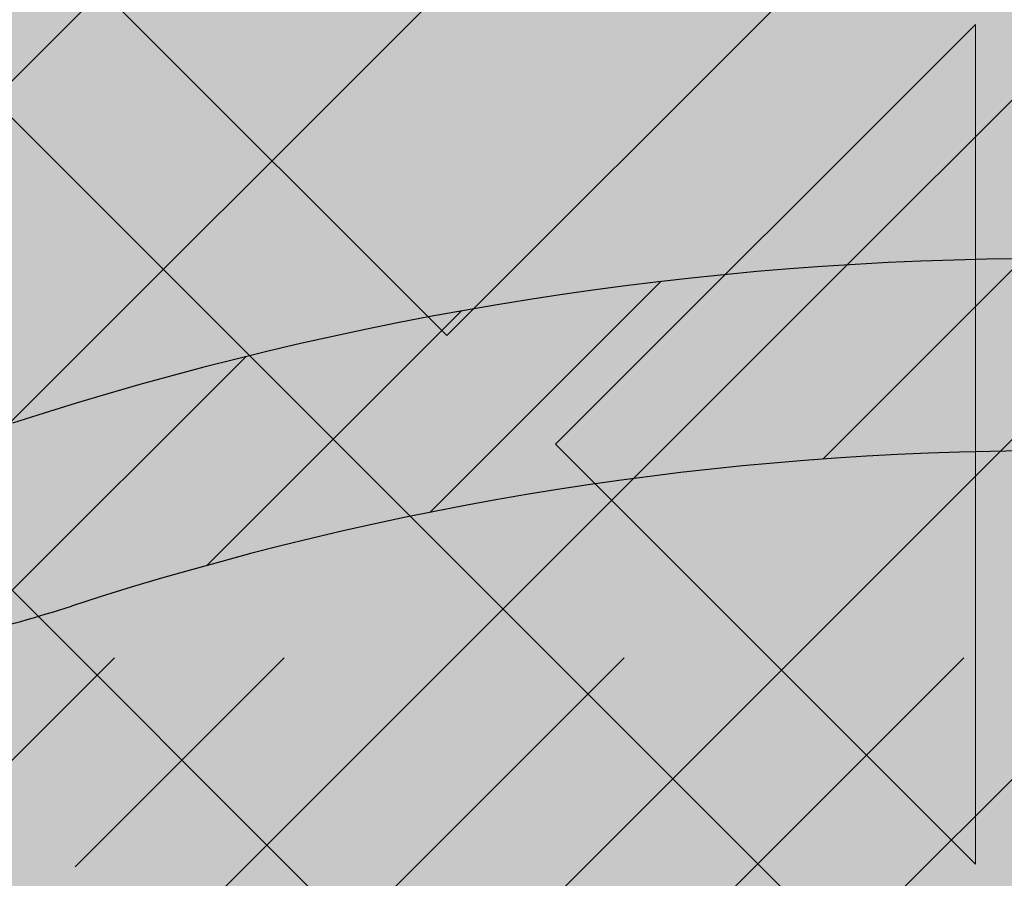
# Model space of a CAD drawing. Units: inches. Extents: x 844 to 2234, y 346 to 1084.
# Tile 20 of 93: x 1121.143 to 1122.777, y 702.178 to 703.603. Entities that reach past the tile are written whole.
import ezdxf

# ---------------------------------------------------------------- set-up
doc = ezdxf.new("R2010")
doc.units = ezdxf.units.IN
doc.header["$MEASUREMENT"] = 0
for name, color, linetype, lineweight in [('A-ANNO-DIMS', 2, 'Continuous', 18), ('furniture', 8, 'Continuous', 18), ('RA-AP-01$0$INT', 35, 'Continuous', 5)]:
    doc.layers.add(name, color=color, linetype=linetype, lineweight=lineweight)
doc.layers.add('RA-AP-01$0$FURN', color=3, linetype='Continuous')
doc.layers.add('RA-AP-01$0$WOOD', color=64, linetype='Continuous')
doc.styles.get("Standard").update_dxf_attribs({"font": 'arial.ttf'})
doc.dimstyles.get("Standard").update_dxf_attribs({"dimtxt": 6, "dimasz": 3, "dimexe": 0.18, "dimexo": 0.0625, "dimgap": 0.09, "dimtad": 0, "dimtih": 1, "dimtoh": 1, "dimdec": 1, "dimzin": 0, "dimdsep": 46, "dimlunit": 3, "dimtxsty": 'Standard', "dimblk": 'ARCHTICK', "dimcen": 0.09, "dimadec": 0, "dimazin": 0, "dimtfac": 1, "dimtdec": 1, "dimtofl": 0, "dimtmove": 0, "dimatfit": 3, "dimfxl": 1, "dimtolj": 1, "dimtzin": 0, "dimarcsym": 0})

# ---------------------------------------------------------------- blocks, each defined once
blk = doc.blocks.new('A$C18D01794')
at = {"layer": 'RA-AP-01$0$INT'}
h = blk.add_hatch(color=256, dxfattribs=at)
h.paths.add_polyline_path([(4.585917135068448, -7.856712009587804), (4.614201406330596, -7.856712009587056), (4.668846067270487, -7.802067348644738), (4.723490728212344, -7.856712009584164), (4.771774999457151, -7.856712009582887), (4.826419660396886, -7.80206734864072), (4.862780050090322, -7.838427738332541), (4.844495778842715, -7.856712009580965), (4.862780050090411, -7.856712009580482), (4.905206456960182, -7.814285602707865), (4.947632863832445, -7.856712009578238), (4.965917135079675, -7.856712009577755), (4.947632863831759, -7.838427738330656), (4.983993253523576, -7.802067348637219), (5.038637914464627, -7.856712009575829), (5.08692218571208, -7.856712009574554), (5.141566846649976, -7.802067348634224), (5.196211507589851, -7.856712009571666), (5.224495778822615, -7.856712009570916), (4.905206456953975, -7.537422687702283)])
h.paths.add_polyline_path([(4.895206456956031, -7.575706958950402), (4.895206456958921, -7.684996280828174), (4.840561796018589, -7.630351619890275)], flags=16)
h.paths.add_polyline_path([(4.915206456955638, -7.575706958949956), (4.969851117895509, -7.630351619887399), (4.915206456957609, -7.684996280827732)], flags=16)
h.paths.add_polyline_path([(4.826419660395175, -7.644493755514321), (4.881064321335613, -7.699138416452331), (4.771774999456703, -7.69913841645522)], flags=16)
h.paths.add_polyline_path([(4.983993253519558, -7.644493755510815), (5.038637914460456, -7.699138416449285), (4.929348592581548, -7.69913841645126)], flags=16)
h.paths.add_polyline_path([(4.881064321336025, -7.719138416452334), (4.826419660397532, -7.773783077393256), (4.771774999457062, -7.719138416455217)], flags=16)
h.paths.add_polyline_path([(4.929348592582019, -7.71913841645126), (5.038637914460982, -7.719138416449284), (4.983993253522945, -7.773783077389749)], flags=16)
h.paths.add_polyline_path([(4.895206456960191, -7.733280552075633), (4.895206456962115, -7.806001331460164), (4.876922185715016, -7.824285602708492), (4.840561796021581, -7.787925213016675)], flags=16)
h.paths.add_polyline_path([(4.915206456958487, -7.733280552075187), (4.969851117899527, -7.787925213013798), (4.933490728206909, -7.824285602708034), (4.9152064569598, -7.806001331461736)], flags=16)
h.paths.add_polyline_path([(4.757632863832376, -7.733280552079264), (4.812277524772842, -7.787925213017304), (4.757632863834348, -7.842569873958233)], flags=16)
h.paths.add_polyline_path([(4.737632863832376, -7.73328055207979), (4.737632863834348, -7.842569873958701), (4.682988202893906, -7.787925213020692)], flags=16)
h.paths.add_polyline_path([(5.05278005008503, -7.733280552072701), (5.052780050087917, -7.842569873951664), (4.998135389146995, -7.787925213013169)], flags=16)
h.paths.add_polyline_path([(5.072780050085024, -7.733280552072333), (5.127424711025931, -7.787925213010806), (5.072780050087916, -7.842569873951244)], flags=16)
h.paths.add_polyline_path([(4.935917135072783, -7.506712009583784), (5.255206456948811, -7.826001331459767), (5.255206456948932, -7.797717060211899), (5.200561796010279, -7.743072399273238), (5.255206456949403, -7.688427738334128), (5.25520645694961, -7.640143467086677), (5.200561796009787, -7.585498806146837), (5.236922185702417, -7.549138416454212), (5.255206456949919, -7.56742268770172), (5.255206456949998, -7.549138416454178), (5.212780050078687, -7.506712009583814), (5.25520645695036, -7.464285602712145), (5.255206456950438, -7.446001331464763), (5.236922185702424, -7.464285602712779), (5.200561796009796, -7.427925213020149), (5.255206456950753, -7.373280552079203), (5.25520645695096, -7.324996280834394), (5.200561796010322, -7.270351619893748), (5.255206456951428, -7.215706958952649), (5.255206456951547, -7.187422687705071)])
h.paths.add_polyline_path([(5.042988202883395, -7.42792521302065), (5.097632863823085, -7.373280552080975), (5.097632863822622, -7.482569873959883)], flags=16)
h.paths.add_polyline_path([(5.028846067259663, -7.442067348644384), (5.083490728198774, -7.496712009583504), (4.974201406321001, -7.496712009583035)], flags=16)
h.paths.add_polyline_path([(5.117632863823087, -7.37328055208089), (5.172277524762331, -7.42792521302015), (5.11763286382262, -7.482569873959851)], flags=16)
h.paths.add_polyline_path([(5.08349072819877, -7.516712009582191), (5.028846067259652, -7.571356670521302), (4.974201406320998, -7.516712009582638)], flags=16)
h.paths.add_polyline_path([(5.131774999446817, -7.35913841645716), (5.186419660386065, -7.413783077396415), (5.241064321325782, -7.359138416456712)], flags=17)
h.paths.add_polyline_path([(5.131774999446228, -7.496712009583703), (5.186419660386065, -7.442067348643883), (5.222780050079488, -7.478427738337313), (5.204495778832781, -7.496712009584014)], flags=16)
h.paths.add_polyline_path([(5.097632863822613, -7.530854145205813), (5.097632863823061, -7.640143467084723), (5.042988202883383, -7.585498806145032)], flags=16)
h.paths.add_polyline_path([(5.131774999446899, -7.339138416457162), (5.241064321325809, -7.339138416456712), (5.186419660386591, -7.284493755517479)], flags=17)
h.paths.add_polyline_path([(5.131774999446226, -7.516712009581999), (5.204495778830767, -7.516712009581702), (5.22278005007868, -7.534996280829206), (5.186419660386049, -7.571356670521828)], flags=16)
h.paths.add_polyline_path([(5.11763286382262, -7.530854145205852), (5.17227752476232, -7.585498806145562), (5.117632863823064, -7.64014346708481)], flags=16)
h.paths.add_polyline_path([(5.186419660386069, -7.599640941770585), (5.241064321325754, -7.654285602710281), (5.131774999446791, -7.654285602709814)], flags=16)
h.paths.add_polyline_path([(5.131774999446872, -7.674285602709813), (5.24106432132578, -7.674285602710282), (5.186419660386554, -7.728930263649504)], flags=16)
h.paths.add_polyline_path([(5.255206456951811, -7.126001331467467), (5.255206456951895, -7.106712009588038), (4.555206456956052, -7.106712009588038), (4.555206456956136, -7.12600133146746), (4.905206456953973, -7.476001331465289)])
h.paths.add_polyline_path([(4.983993253513404, -7.368930263651977), (4.92934859257295, -7.314285602713969), (5.03863791445186, -7.314285602711063)], flags=16)
h.paths.add_polyline_path([(4.969851117889988, -7.383072399276016), (4.915206456952556, -7.437717060215906), (4.915206456949648, -7.328427738338133)], flags=16)
h.paths.add_polyline_path([(4.929348592572535, -7.294285602713971), (4.983993253511019, -7.239640941773039), (5.038637914451496, -7.294285602711065)], flags=16)
h.paths.add_polyline_path([(5.052780050074912, -7.280143467087016), (4.998135389134438, -7.225498806148989), (5.052780050072919, -7.170854145208052)], flags=16)
h.paths.add_polyline_path([(5.07278005007491, -7.280143467086489), (5.072780050072918, -7.170854145207579), (5.127424711013374, -7.225498806145578)], flags=16)
h.paths.add_polyline_path([(4.89520645695295, -7.437717060216355), (4.840561796013067, -7.383072399278919), (4.895206456950961, -7.328427738338582)], flags=16)
h.paths.add_polyline_path([(4.915206456948365, -7.280143467090674), (4.915206456946434, -7.207422687704125), (4.933490728192729, -7.18913841645701), (4.969851117886972, -7.225498806149623)], flags=16)
h.paths.add_polyline_path([(4.881064321327021, -7.314285602715054), (4.82641966038902, -7.368930263655506), (4.771774999448108, -7.314285602717047)], flags=16)
h.paths.add_polyline_path([(4.895206456950073, -7.280143467091125), (4.840561796009022, -7.225498806152518), (4.876922185700835, -7.18913841645908), (4.895206456948749, -7.207422687706589)], flags=16)
h.paths.add_polyline_path([(4.983993253510392, -7.211356670525576), (4.947632863816944, -7.174996280833758), (4.965917135064043, -7.156712009585847), (5.038637914448995, -7.156712009584522)], flags=16)
h.paths.add_polyline_path([(4.881064321326543, -7.294285602715056), (4.771774999447578, -7.294285602717046), (4.826419660385607, -7.239640941776569)], flags=16)
h.paths.add_polyline_path([(4.905206456946447, -7.19913841645844), (4.862780050074785, -7.156712009587725), (4.947632863816685, -7.156712009586302)], flags=16)
h.paths.add_polyline_path([(5.14156684663679, -7.211356670521528), (5.086922185696452, -7.156712009583639), (5.196211507574223, -7.156712009581651)], flags=16)
h.paths.add_polyline_path([(4.8264196603837, -7.211356670529104), (4.771774999442643, -7.156712009590501), (4.8444957788276, -7.156712009588568), (4.862780050075511, -7.17499628083566)], flags=16)
h.paths.add_polyline_path([(4.812277524760289, -7.225498806153156), (4.757632863822258, -7.28014346709363), (4.757632863819352, -7.170854145214669)], flags=16)
h.paths.add_polyline_path([(4.73763286382226, -7.280143467093997), (4.682988202881349, -7.22549880615554), (4.737632863819352, -7.170854145215086)], flags=16)
h.paths.add_polyline_path([(4.723490728195188, -7.156712009591787), (4.668846067257299, -7.211356670532127), (4.614201406317417, -7.156712009594693)], flags=16)
h.paths.add_polyline_path([(4.597632863829262, -7.506712009583814), (4.555206456957951, -7.54913841645418), (4.555206456958029, -7.56742268770172), (4.573490728205535, -7.549138416454212), (4.609851117898167, -7.585498806146839), (4.555206456958338, -7.640143467086675), (4.555206456958546, -7.688427738334125), (4.60985111789767, -7.743072399273238), (4.555206456959015, -7.797717060211899), (4.555206456959138, -7.826001331459767), (4.874495778835167, -7.506712009583786), (4.5552064569564, -7.187422687705062), (4.555206456956523, -7.215706958952644), (4.609851117897629, -7.270351619893746), (4.555206456956988, -7.324996280834396), (4.555206456957198, -7.373280552079195), (4.609851117898153, -7.427925213020147), (4.573490728205528, -7.464285602712779), (4.555206456957507, -7.446001331464756), (4.555206456957585, -7.464285602712143)])
h.paths.add_polyline_path([(4.712780050085332, -7.482569873959882), (4.712780050084863, -7.373280552080972), (4.767424711024555, -7.42792521302065)], flags=16)
h.paths.add_polyline_path([(4.726922185709173, -7.496712009583504), (4.781566846648288, -7.442067348644384), (4.836211507586949, -7.496712009583033)], flags=16)
h.paths.add_polyline_path([(4.692780050085327, -7.482569873959851), (4.638135389145619, -7.427925213020149), (4.692780050084865, -7.373280552080892)], flags=16)
h.paths.add_polyline_path([(4.726922185709182, -7.516712009582191), (4.836211507586949, -7.51671200958264), (4.7815668466483, -7.571356670521304)], flags=16)
h.paths.add_polyline_path([(4.678637914461726, -7.496712009583706), (4.605917135075169, -7.496712009584014), (4.587632863828464, -7.478427738337311), (4.623993253521887, -7.442067348643881)], flags=16)
h.paths.add_polyline_path([(4.712780050085336, -7.530854145205816), (4.767424711024568, -7.585498806145034), (4.71278005008489, -7.640143467084724)], flags=16)
h.paths.add_polyline_path([(4.678637914461726, -7.516712009582001), (4.623993253521899, -7.571356670521829), (4.587632863829271, -7.534996280829206), (4.605917135077185, -7.5167120095817)], flags=16)
h.paths.add_polyline_path([(4.692780050085336, -7.530854145205848), (4.692780050084889, -7.64014346708481), (4.638135389145632, -7.585498806145562)], flags=16)
h.paths.add_polyline_path([(4.623993253521885, -7.413783077396415), (4.678637914461131, -7.359138416457161), (4.56934859258217, -7.359138416456712)], flags=17)
h.paths.add_polyline_path([(4.623993253521901, -7.599640941770568), (4.678637914461158, -7.654285602709814), (4.569348592582195, -7.654285602710281)], flags=16)
h.paths.add_polyline_path([(4.678637914461051, -7.339138416457162), (4.623993253521361, -7.284493755517479), (4.569348592582143, -7.339138416456712)], flags=17)
h.paths.add_polyline_path([(4.678637914461076, -7.674285602709813), (4.623993253521399, -7.728930263649504), (4.569348592582167, -7.674285602710281)], flags=16)
h = blk.add_hatch(color=256, dxfattribs=at)
h.paths.add_polyline_path([(4.905206456954232, -7.537422687702028), (4.874495778835232, -7.506712009583718), (4.555206456959138, -7.826001331459766), (4.555206456959269, -7.856712009588616), (4.585917135068449, -7.856712009587804)])
h.paths.add_polyline_path([(4.935917135072152, -7.506712009583152), (4.905206456953497, -7.537422687701806), (5.224495778822614, -7.856712009570917), (5.255206456948681, -7.856712009570104), (5.255206456948813, -7.826001331459768)])
h.paths.add_polyline_path([(5.255206456951549, -7.18742268770507), (5.255206456951813, -7.126001331467461), (4.905206456953563, -7.476001331465701), (4.935917135072559, -7.506712009584006)])
h.paths.add_polyline_path([(4.874495778835167, -7.506712009583785), (4.905206456953818, -7.476001331465132), (4.555206456956135, -7.126001331467458), (4.555206456956399, -7.187422687705064)])
h = blk.add_hatch(color=256, dxfattribs=at)
h.paths.add_polyline_path([(4.969851117891331, -7.630351619889621), (4.915206456952669, -7.575706958950966), (4.915206456952222, -7.684996280828739)])
h.paths.add_polyline_path([(4.895206456953064, -7.575706958950968), (4.840561796014413, -7.630351619889628), (4.895206456953533, -7.684996280828741)])
h.paths.add_polyline_path([(4.826419660390684, -7.644493755513362), (4.771774999451003, -7.699138416453052), (4.881064321329913, -7.699138416452587)])
h.paths.add_polyline_path([(4.881064321329884, -7.719138416452585), (4.771774999450921, -7.719138416453052), (4.82641966039018, -7.773783077392298)])
h.paths.add_polyline_path([(4.895206456953734, -7.733280552076196), (4.840561796013912, -7.787925213016031), (4.876922185707337, -7.824285602709455), (4.895206456954043, -7.806001331462747)])
h.paths.add_polyline_path([(4.862780050082808, -7.838427738332388), (4.826419660390178, -7.802067348639763), (4.771774999450351, -7.856712009579595), (4.844495778835303, -7.856712009579895)])
h.paths.add_polyline_path([(4.812277524766446, -7.787925213016036), (4.757632863827191, -7.733280552076788), (4.757632863826741, -7.842569873955747)])
h.paths.add_polyline_path([(4.737632863827191, -7.733280552076863), (4.682988202887508, -7.787925213016558), (4.737632863826743, -7.842569873955778)])
h.paths.add_polyline_path([(4.668846067263777, -7.802067348640287), (4.614201406325123, -7.856712009578949), (4.723490728202894, -7.856712009579402)])
h.paths.add_polyline_path([(4.905206456953846, -7.814285602708654), (4.862780050082654, -7.856712009579847), (4.947632863824561, -7.85671200958032)])
h.paths.add_polyline_path([(4.915206456952028, -7.733280552076195), (4.91520645695173, -7.806001331460731), (4.933490728199234, -7.824285602708648), (4.96985111789186, -7.787925213016022)])
h.paths.add_polyline_path([(5.038637914454841, -7.719138416453029), (4.929348592575874, -7.71913841645258), (4.983993253515593, -7.773783077392289)])
h.paths.add_polyline_path([(4.983993253515065, -7.644493755513352), (4.929348592575849, -7.699138416452582), (5.038637914454755, -7.699138416453031)])
h.paths.add_polyline_path([(5.052780050079843, -7.73328055207676), (4.998135389140595, -7.787925213016018), (5.052780050080309, -7.842569873955721)])
h.paths.add_polyline_path([(4.983993253516868, -7.802067348639752), (4.947632863824241, -7.838427738332383), (4.965917135071747, -7.856712009579888), (5.038637914456701, -7.856712009579572)])
h.paths.add_polyline_path([(5.127424711019533, -7.787925213016519), (5.072780050079843, -7.733280552076838), (5.07278005008031, -7.842569873955751)])
h.paths.add_polyline_path([(5.141566846643269, -7.802067348640248), (5.086922185704154, -7.85671200957937), (5.196211507581929, -7.856712009578901)])
for p, q in [((4.874495778835167, -7.506712009583786), (4.555206456959136, -7.826001331459769)), ((4.905206456953975, -7.537422687702283), (4.585917135071132, -7.856712009585121)), ((4.895206456956031, -7.575706958950402), (4.840561796018589, -7.630351619890275)), ((4.895206456958921, -7.684996280828173), (4.895206456956031, -7.575706958950402)), ((4.895206456958917, -7.684996280828171), (4.840561796018589, -7.630351619890275)), ((4.826419660395171, -7.644493755514321), (4.771774999456703, -7.69913841645522)), ((4.881064321335613, -7.699138416452333), (4.826419660395173, -7.64449375551432))]:
    blk.add_line(p, q, dxfattribs=at)
blk = doc.blocks.new('A$C32926AE1')
at = {"layer": 'RA-AP-01$0$FURN'}
h = blk.add_hatch(dxfattribs=at)
h.set_pattern_fill('ANSI31', color=256, scale=0.1, style=0)
h.set_pattern_definition([(45, (0, 0), (-0.0088388347648318, 0.0088388347648318), [])])
edge = h.paths.add_edge_path(flags=16)
edge.add_arc((4.904771284329206, 4.246793130718756), 0.2603971832811541, 75.22398030683196, 104.7760196931204)
edge.add_arc((4.904771284329206, 4.246793130718756), 0.2603971832811541, 75.223980306832, 104.77601969312039, ccw=False)
edge = h.paths.add_edge_path(flags=16)
edge.add_arc((4.904771284329206, 4.067062675376612), 0.2603971832811541, 255.2239803068796, 284.776019693168)
edge.add_arc((4.904771284329206, 4.067062675376612), 0.2603971832811541, 255.22398030687958, 284.77601969316805, ccw=False)
edge = h.paths.add_edge_path(flags=0)
edge.add_arc((4.904771284329206, 4.067062675376612), 0.2603971832811541, 255.2239803068796, 284.776019693168)
edge.add_arc((4.904771284329206, 4.067062675376612), 0.2603971832811541, 255.22398030687958, 284.77601969316805, ccw=False)
edge = h.paths.add_edge_path(flags=0)
edge.add_arc((4.904771284329206, 4.067062675376612), 0.2603971832811541, 255.2239803068796, 284.776019693168)
edge.add_arc((4.904771284329206, 4.067062675376612), 0.2603971832811541, 255.22398030687958, 284.77601969316805, ccw=False)
edge = h.paths.add_edge_path()
edge.add_arc((4.604388392048174, 4.588829985554312), 0.1599999999999918, 342.3781640246255, 354.4317409793762)
edge.add_arc((5.090145208887507, 4.43216705527679), 0.3503971832811637, 162.0091218307731, 180.3186872093483)
edge.add_arc((5.205154176610243, 4.588829985554953), 0.1599999999999917, 185.5682590208461, 197.6218359767349)
edge.add_arc((4.904771284329229, 4.246793130718735), 0.3503971832811761, 72.00912183053516, 107.9908781690354)
edge.add_arc((9.535952835716557, 4.28682295566602), 4.798342501046485, 178.2875002453811, 181.5576802719453)
edge.add_arc((4.719397359771122, 4.43216705527679), 0.3503971832811637, 359.6813127906516, 377.9908781692269)
edge.add_arc((9.535967292294904, 4.286822350292874), 4.778371420254705, 178.2965938931842, 181.5667745797229)
edge.add_arc((4.719397359771122, 4.43216705527679), 0.3303971832811637, 359.6813127906516, 377.9908781692269)
edge.add_arc((0.2735752763637294, 4.286822350292874), 4.7783714202547, 358.4332254202771, 361.7034061068158)
edge.add_arc((5.061434214606998, 4.732549947558029), 0.1600000000000254, 252.3781640250584, 264.4317409792362)
edge.add_arc((4.748108354051257, 4.732549947558012), 0.1600000000000541, 275.5682590208426, 287.6218359759532)
edge.add_arc((4.604388392048115, 4.588829985554317), 0.1800000000000505, 342.3567572500182, 349.3735009646207)
edge.add_arc((5.205154176610254, 4.588829985554976), 0.1800000000000069, 190.6264990356027, 197.6432427513933)
edge.add_arc((5.061434214607106, 4.732549947558013), 0.1800000000000424, 252.3567572496606, 259.3735009644582)
edge.add_arc((4.904771284329208, 4.246793130718737), 0.3303971832811676, 71.99844483668534, 108.0015551637021)
edge.add_arc((4.748108354051414, 4.732549947558045), 0.1800000000000547, 280.6264990355479, 287.6432427495938)
edge.add_arc((5.090145208887514, 4.432167055276789), 0.2803971832811691, 162.8706300666893, 180.816523289902)
edge.add_arc((4.719397359771136, 4.432167055276689), 0.2803971832811534, 359.183476710103, 377.1293699333214)
edge.add_arc((4.904771284329222, 4.246793130718737), 0.2803971832811769, 72.87063006672916, 107.1293699332334)
edge.add_arc((5.090145208887522, 4.432167055276788), 0.2603971832811776, 165.2239803068007, 180.9953123810312)
edge.add_arc((4.719397359771141, 4.432167055276699), 0.2603971832811458, 359.0046876189768, 374.7760196932087)
edge.add_arc((5.090145208887507, 4.43216705527679), 0.3303971832811637, 162.0091218307731, 180.3186872093483)
edge.add_arc((9.53595427642584, 4.285015535491528), 4.728345371032053, 178.265043920078, 181.5679956281801)
edge.add_arc((0.2735882922327999, 4.285015535491582), 4.728345371032045, 358.4320043718193, 361.7349560799204)
edge.add_arc((9.535953591267507, 4.284458026472751), 4.708343996644348, 178.2573054306777, 181.5704995759608)
edge.add_arc((0.273588977391114, 4.284458026472785), 4.708343996644358, 358.4295004240388, 361.7426945693213)
edge.add_arc((0.2735889773911131, 4.029397779622582), 4.708343996644359, 358.2573054306787, 361.5704995759613)
edge.add_arc((9.535953591267518, 4.029397779622618), 4.708343996644359, 178.4295004240391, 181.7426945693223)
edge.add_arc((0.2735882922327901, 4.028840270603786), 4.728345371032054, 358.2650439200796, 361.5679956281808)
edge.add_arc((9.53595427642584, 4.028840270603841), 4.728345371032054, 178.4320043718199, 181.7349560799219)
edge.add_arc((0.2735752763637302, 4.027033455802493), 4.778371420254699, 358.2965938931842, 361.5667745797229)
edge.add_arc((4.719397359771122, 3.881688750818578), 0.3303971832811637, 342.0091218307731, 360.3186872093484)
edge.add_arc((5.090145208887507, 3.881688750818578), 0.3303971832811637, 179.6813127906516, 197.9908781692269)
edge.add_arc((9.535967292294904, 4.027033455802493), 4.778371420254705, 178.433225420277, 181.7034061068158)
edge.add_arc((4.719397359771122, 3.881688750818578), 0.3503971832811637, 342.0091218307731, 360.3186872093484)
edge.add_arc((9.53595283571655, 4.027032850429349), 4.79834250104648, 178.4423197280546, 181.7124997546188)
edge.add_arc((4.719397359771141, 3.881688750818669), 0.2603971832811458, 345.2239803067913, 360.9953123810232)
edge.add_arc((5.090145208887522, 3.88168875081858), 0.2603971832811776, 179.0046876189687, 194.7760196931993)
edge.add_arc((4.904771284329222, 4.067062675376631), 0.2803971832811769, 252.8706300667665, 287.1293699332708)
edge.add_arc((4.719397359771136, 3.881688750818678), 0.2803971832811534, 342.8706300666787, 360.8165232898969)
edge.add_arc((5.090145208887514, 3.881688750818579), 0.2803971832811691, 179.183476710098, 197.1293699333106)
edge.add_arc((4.748108354051414, 3.581305858537323), 0.1800000000000547, 72.3567572504062, 79.37350096445199)
edge.add_arc((4.904771284329208, 4.067062675376631), 0.3303971832811676, 251.9984448362979, 288.0015551633146)
edge.add_arc((5.061434214607106, 3.581305858537355), 0.1800000000000424, 100.6264990355418, 107.6432427503394)
edge.add_arc((5.205154176610254, 3.725025820540392), 0.1800000000000069, 162.3567572486066, 169.3735009643972)
edge.add_arc((4.604388392048115, 3.725025820541051), 0.1800000000000505, 10.62649903537925, 17.64324274998182)
edge.add_arc((4.748108354051257, 3.581305858537356), 0.1600000000000541, 72.37816402404681, 84.43174097915735)
edge.add_arc((4.904771284329229, 4.067062675376632), 0.3503971832811761, 252.0091218309645, 287.9908781694648)
edge.add_arc((5.061434214606998, 3.581305858537339), 0.1600000000000254, 95.56825902076373, 107.6218359749416)
edge.add_arc((5.205154176610243, 3.725025820540414), 0.1599999999999917, 162.3781640232651, 174.4317409791539)
edge.add_arc((5.090145208887507, 3.881688750818578), 0.3503971832811637, 179.6813127906516, 197.9908781692269)
edge.add_arc((4.604388392048174, 3.725025820541056), 0.1599999999999918, 5.568259020623824, 17.62183597537444)
edge.add_arc((0.2735897329420762, 4.28682295566602), 4.798342501046482, 358.4423197280547, 361.7124997546188)
edge.add_arc((0.2735897329420691, 4.027032850429348), 4.798342501046489, 358.2875002453812, 361.5576802719453)
at = {"layer": 'RA-AP-01$0$WOOD'}
h = blk.add_hatch(color=256, dxfattribs=at)
h.dxf.hatch_style = 1
h.paths.add_polyline_path([(5.157430609644524, 4.573483066760929, -0.1009492694046607), (5.155401577623758, 4.593365984175333, -0.1842662638101597), (5.172249623284174, 4.638795604568598, 0.2056608120311276), (5.179560981299304, 4.661316324430096, 0.3614336704623542), (5.134352340494423, 4.706524965234944, 0.2056608120311297), (5.111831620632933, 4.699213607219793, -0.1842662638101113), (5.066402000239693, 4.682365561559342, -0.1055311479399994), (5.045656153913092, 4.68467289944697, 0.1567636581983829), (4.763886414745334, 4.684672899446966, -0.1055311479399895), (4.743140568418733, 4.68236556155934, -0.1842662638100833), (4.6977109480255, 4.69921360721979, 0.2056608120302612), (4.675190228164109, 4.706524965234949, 0.3614336704708441), (4.629981587358889, 4.66131632442871, 0.2056608120245944), (4.637292945374126, 4.638795604567974, -0.1842662638101024), (4.654140991034615, 4.59336598417475, -0.1009492694055169), (4.652111959013835, 4.573483066760181, 0.021410119221476), (4.629748025606143, 4.156712009541676, 0.0214101192214795), (4.652111959013809, 3.739940952323101, -0.1009492694059586), (4.654140991034615, 3.720058034908448, -0.1842662638100975), (4.637292945374126, 3.674628414515226, 0.2056608120245705), (4.629981587358889, 3.652107694654492, 0.3614336704708879), (4.675190228164113, 3.606899053848249, 0.2056608120302384), (4.697710948025501, 3.614210411863408, -0.1842662638100995), (4.743140568418738, 3.63105845752386, -0.1055311479402541), (4.763886414745388, 3.628751119636215, 0.1567636581983776), (5.045656153913137, 3.628751119636244, -0.1055311479397538), (5.066402000239692, 3.631058457523857, -0.1842662638101067), (5.111831620632931, 3.614210411863407, 0.2056608120310924), (5.134352340494417, 3.606899053848256, 0.3614336704624001), (5.179560981299307, 3.652107694653103, 0.2056608120311314), (5.172249623284175, 3.6746284145146, -0.1842662638101402), (5.155401577623758, 3.72005803490786, -0.1009492694051366), (5.15743060964455, 3.739940952322354, 0.0214101192215073), (5.179794543052287, 4.156712009541468, 0.0214101192215252)])
h.paths.add_polyline_path([(4.639748609479751, 4.156712009541513, 0.0213537860821624), (4.661970494867118, 3.741887061152232, -0.094075836301374), (4.664143710413708, 3.7196126951003, -0.1824818158568985), (4.644813765429836, 3.668037719127816, 0.2056608120245319), (4.639939526753007, 3.653023905887301, 0.3614336704710246), (4.676106439397173, 3.616856993242342, 0.2056608120302234), (4.691120252638095, 3.621731231919122, -0.1824818158602558), (4.742695228611606, 3.641061176902986, -0.1029891339458722), (4.766991894714349, 3.638256818950944, 0.156709409989566), (5.042550673941472, 3.638256818950105, -0.102989133958497), (5.066847340047078, 3.641061176902949, -0.1824818158594995), (5.118422316020358, 3.621731231919103, 0.2056608120311416), (5.133436129261316, 3.616856993242346, 0.3614336704621468), (5.169603041905217, 3.653023905886178, 0.2056608120310986), (5.164728803228477, 3.668037719127177, -0.1824818158565612), (5.145398858244737, 3.719612695099578, -0.0940758363009313), (5.147572073791232, 3.741887061151398, 0.0213537860822023), (5.169793959178681, 4.156712009541451, 0.0213537860822226), (5.147572073791203, 4.571536957931898, -0.0940758363005034), (5.145398858244737, 4.59381132398362, -0.1824818158565587), (5.164728803228476, 4.645386299956021, 0.2056608120311045), (5.169603041905216, 4.66040011319702, 0.3614336704621845), (5.133436129261313, 4.696567025840856, 0.2056608120310773), (5.118422316020359, 4.691692787164098, -0.182481815859508), (5.066847340047078, 4.67236284218025, -0.1029891339584606), (5.04255067394148, 4.675167200133092, 0.156709409989566), (4.766991894714357, 4.675167200132257, -0.1029891339458842), (4.742695228611611, 4.672362842180213, -0.1824818158602725), (4.691120252638095, 4.691692787164077, 0.2056608120302152), (4.676106439397174, 4.696567025840858, 0.3614336704710363), (4.639939526753005, 4.660400113195899, 0.2056608120245495), (4.644813765429837, 4.645386299955384, -0.1824818158568934), (4.664143710413708, 4.593811323982902, -0.0940758363009187), (4.661970494867149, 4.571536957931074, 0.021353786082177)], flags=16)
h.paths.add_polyline_path([(5.129794543052235, 4.432167055276933, -0.0141661062790638), (5.130152669293814, 4.156927903047693, -0.0141661062790647), (5.129794543052234, 3.881688750818433, -0.0785247771143638), (5.10979738006795, 3.755143611847103, 0.0945969212073497), (5.105408519571111, 3.717898134952927, 0.1043170707844957), (5.116074640131521, 3.670385395016088, 0.1043170707864965), (5.068561900193738, 3.681051515576561, 0.09459692119553), (5.031316423304057, 3.676662655080835, -0.1580239521427272), (4.778226145355827, 3.676662655080367, 0.0945969211986668), (4.740980668464973, 3.681051515576592, 0.1043170707882822), (4.693467928526415, 3.670385395015844, 0.1043170707867916), (4.704134049087309, 3.717898134953662, 0.0945969211972894), (4.69974518859162, 3.755143611844042, -0.0785247771163196), (4.679748025606343, 3.881688750818406, -0.0141661062790663), (4.679389899364763, 4.156927903047693, -0.0141661062790672), (4.679748025606343, 4.432167055276998, -0.0785247771163064), (4.699745188591625, 4.55871219425134, 0.094596921197333), (4.704134049087308, 4.595957671141738, 0.1043170707867205), (4.693467928526416, 4.643470411079523, 0.1043170707882628), (4.740980668464965, 4.632804290518776, 0.0945969211988114), (4.778226145355874, 4.637193151015016, -0.158023952142669), (5.031316423304015, 4.637193151014546, 0.0945969211956361), (5.068561900193736, 4.632804290518806, 0.1043170707864979), (5.11607464013152, 4.643470411079278, 0.1043170707844617), (5.105408519571112, 4.595957671142455, 0.0945969212074597), (5.109797380067959, 4.558712194248236, -0.0785247771143467)], flags=0)
h.paths.add_polyline_path([(5.119794532311105, 4.432259799204851, -0.0142000800617244), (5.120156169157484, 4.156927903047701, -0.0142000800617277), (5.119794532311105, 3.881596006890482, -0.0784894509520253), (5.100273383573699, 3.758192358677797, 0.0940138827242913), (5.095413455884425, 3.717477693979438, 0.0606271852308753), (5.099615656341024, 3.686844378806616, 0.0606271852322524), (5.068982341167493, 3.691046579263239, 0.0940138827010453), (5.028267676478798, 3.686186651576848, -0.1580706864508061), (4.781274892180912, 3.686186651576435, 0.0940138827026903), (4.740560227491556, 3.691046579263279, 0.0606271852339895), (4.709926912317155, 3.686844378806508, 0.0606271852329405), (4.714129112773991, 3.717477693980356, 0.094013882701304), (4.709269185087677, 3.758192358669163, -0.0784894509577193), (4.689748036347473, 3.881596006890469, -0.014200080061729), (4.689386399501094, 4.156927903047709, -0.0142000800617217), (4.689748036347473, 4.432259799204808, -0.078489450957724), (4.709269185087651, 4.555663447426125, 0.0940138827014585), (4.714129112773992, 4.596378112114996, 0.0606271852329731), (4.709926912317154, 4.62701142728886, 0.0606271852340196), (4.74056022749157, 4.622809226832087, 0.0940138827024997), (4.781274892180847, 4.627669154518912, -0.1580706864508359), (5.028267676478777, 4.627669154518526, 0.0940138827010946), (5.068982341167492, 4.622809226832129, 0.060627185232254), (5.099615656341024, 4.627011427288751, 0.0606271852308727), (5.095413455884425, 4.59637811211593, 0.0940138827241088), (5.100273383573675, 4.555663447417647, -0.0784894509520978)], flags=0)
h.paths.add_polyline_path([(5.06978912287499, 4.430218106756144, -0.014241683694547), (5.070173729147532, 4.156927903047672, -0.0142416836945458), (5.06978912287499, 3.883637699339223, -0.0800609523125196), (5.052662118612511, 3.773463122773442, 0.0526421978001116), (5.04590916754064, 3.740550867606997, 0.0526421977992423), (5.012996912374707, 3.73379791653534, -0.1583028414718258), (4.796545656286308, 3.73379791653451, 0.0526421978034211), (4.763633401117837, 3.740550867607021, 0.0526421978018622), (4.756880450045755, 3.773463122774558, -0.0800609523117106), (4.739753445783639, 3.883637699339268, -0.0142416836945435), (4.739368839511098, 4.156927903047671, -0.0142416836945477), (4.739753445783639, 4.430218106756155, -0.0800609523116345), (4.75688045004574, 4.540392683320762, 0.052642197801941), (4.763633401117837, 4.573304938488346, 0.0526421978035071), (4.796545656286361, 4.580057889560873, -0.1583028414717561), (5.012996912374669, 4.580057889560039, 0.0526421977993048), (5.04590916754064, 4.57330493848837, 0.0526421978002057), (5.052662118612529, 4.540392683321868, -0.080060952312477)], flags=0)
h.paths.add_polyline_path([(5.049789715110557, 4.43038092723357, -0.0143097550741839), (5.05018085590259, 4.156927903047715, -0.0143097550741854), (5.049789715110558, 3.883474878861827, -0.0800685599149176), (5.03362098255317, 3.779581877367999, 0.0306258898956367), (5.028241146483733, 3.758218888663947, 0.0306258898977031), (5.006878157778253, 3.75283905259408, -0.1583983521624096), (4.802664410878162, 3.752839052594731, 0.0306258898946014), (4.781301422174808, 3.758218888663924, 0.0306258898967912), (4.775921586105202, 3.779581877368794, -0.080068559914251), (4.759752853548071, 3.883474878861786, -0.0143097550741854), (4.759361712756037, 4.156927903047671, -0.0143097550741854), (4.759752853548071, 4.430380927233557, -0.0800685599142479), (4.775921586105193, 4.534273928726546, 0.0306258898968306), (4.781301422174808, 4.555636917431444, 0.0306258898945754), (4.802664410878143, 4.561016753500631, -0.1583983521624168), (5.006878157778244, 4.561016753501291, 0.0306258898977177), (5.028241146483733, 4.555636917431421, 0.0306258898958182), (5.03362098255321, 4.534273928727244, -0.080068559914796)], flags=0)
h.paths.add_polyline_path([(4.999766070382627, 4.428171244713864, -0.0143443147609634), (5.000198441819402, 4.156927903047689, -0.0143443147609612), (4.999766070382627, 3.885684561381556, -0.0784641635803329), (4.987356730658798, 3.799103304488872, -0.1506053783831347), (4.822185837999821, 3.79910330448882, -0.0784641635803318), (4.809776498276007, 3.885684561381509, -0.014344314760963), (4.809344126839227, 4.156927903047677, -0.0143443147609645), (4.809776498276007, 4.428171244713873, -0.0784641635803192), (4.822185837999822, 4.514752501606549, -0.1506053783831338), (4.987356730658798, 4.514752501606494, -0.078464163580285)], flags=0)
h.paths.add_polyline_path([(4.979755254238824, 4.42764379880488, -0.0143772539198268), (4.980205517789977, 4.156927903047693, -0.0143772539198275), (4.979755254238824, 3.886212007290489, -0.0689242507424422), (4.971183264704897, 3.815276770442801, -0.1296645318904179), (4.838359303953726, 3.815276770442746, -0.0689242507424186), (4.829787314419809, 3.886212007290419, -0.0143772539198292), (4.829337050868653, 4.156927903047653, -0.0143772539198325), (4.829787314419809, 4.427643798804946, -0.0689242507424211), (4.838359303953725, 4.498579035652621, -0.1296645318904187), (4.971183264704897, 4.498579035652565, -0.0689242507424401)], flags=0)
h = blk.add_hatch(color=256, dxfattribs=at)
h.dxf.hatch_style = 1
h.paths.add_polyline_path([(5.145398858244737, 4.59381132398362, -0.1824818158565616), (5.164728803228476, 4.645386299956021, 0.2056608120311045), (5.169603041905216, 4.66040011319702, 0.3614336704621845), (5.133436129261313, 4.696567025840856, 0.2056608120310773), (5.118422316020359, 4.691692787164098, -0.182481815859508), (5.066847340047078, 4.67236284218025, -0.1029891339584606), (5.04255067394148, 4.675167200133092, 0.156709409989566), (4.766991894714357, 4.675167200132257, -0.1029891339458842), (4.742695228611611, 4.672362842180213, -0.1824818158602725), (4.691120252638095, 4.691692787164077, 0.2056608120302152), (4.676106439397174, 4.696567025840858, 0.3614336704710363), (4.639939526753005, 4.660400113195899, 0.2056608120245495), (4.644813765429837, 4.645386299955384, -0.1824818158568934), (4.664143710413708, 4.593811323982902, -0.0940758363009187), (4.661970494867149, 4.571536957931074, 0.0213537860821772), (4.639748609479751, 4.156712009541507, 0.0213537860821625), (4.661970494867119, 3.741887061152226, -0.0940758363013071), (4.664143710413708, 3.719612695100309, -0.1824818158569294), (4.644813765429836, 3.668037719127816, 0.2056608120245319), (4.639939526753007, 3.653023905887301, 0.3614336704710246), (4.676106439397173, 3.616856993242342, 0.2056608120302234), (4.691120252638095, 3.621731231919122, -0.1824818158602558), (4.742695228611606, 3.641061176902986, -0.1029891339458722), (4.766991894714349, 3.638256818950944, 0.156709409989566), (5.042550673941472, 3.638256818950105, -0.102989133958497), (5.066847340047078, 3.641061176902949, -0.1824818158594995), (5.118422316020358, 3.621731231919103, 0.2056608120311416), (5.133436129261316, 3.616856993242346, 0.3614336704621468), (5.169603041905217, 3.653023905886178, 0.2056608120310986), (5.164728803228477, 3.668037719127177, -0.1824818158565612), (5.145398858244737, 3.719612695099578, -0.0940758363009313), (5.147572073791232, 3.741887061151398, 0.0213537860822023), (5.169793959178681, 4.156712009541451, 0.0213537860822226), (5.147572073791203, 4.571536957931898, -0.0940758363004996)])
h.paths.add_polyline_path([(5.109797380067958, 4.55871219424824, -0.0785247771143472), (5.129794543052234, 4.432167055276936, -0.0141661062790644), (5.130152669293814, 4.156927903047685, -0.014166106279066), (5.129794543052234, 3.881688750818401, -0.0785247771143517), (5.109797380067946, 3.755143611847092, 0.0945969212073132), (5.105408519571111, 3.717898134952929, 0.1043170707844995), (5.116074640131521, 3.670385395016088, 0.1043170707864965), (5.068561900193738, 3.681051515576561, 0.09459692119553), (5.031316423304057, 3.676662655080835, -0.1580239521427272), (4.778226145355827, 3.676662655080367, 0.0945969211986668), (4.740980668464973, 3.681051515576592, 0.1043170707882822), (4.693467928526415, 3.670385395015844, 0.1043170707867916), (4.704134049087309, 3.717898134953662, 0.0945969211972894), (4.69974518859162, 3.755143611844042, -0.0785247771163196), (4.679748025606343, 3.881688750818406, -0.0141661062790663), (4.679389899364763, 4.156927903047693, -0.0141661062790672), (4.679748025606343, 4.432167055276998, -0.0785247771163064), (4.699745188591625, 4.55871219425134, 0.094596921197333), (4.704134049087308, 4.595957671141738, 0.1043170707867205), (4.693467928526416, 4.643470411079523, 0.1043170707882628), (4.740980668464965, 4.632804290518776, 0.0945969211988114), (4.778226145355874, 4.637193151015016, -0.158023952142669), (5.031316423304015, 4.637193151014546, 0.0945969211956361), (5.068561900193736, 4.632804290518806, 0.1043170707864979), (5.11607464013152, 4.643470411079278, 0.1043170707844617), (5.105408519571112, 4.595957671142455, 0.0945969212074504)], flags=16)
h.paths.add_polyline_path([(5.100273383573655, 4.55566344741771, -0.0784894509521388), (5.119794532311105, 4.432259799204852, -0.0142000800617252), (5.120156169157484, 4.156927903047686, -0.014200080061726), (5.119794532311105, 3.881596006890502, -0.0784894509520446), (5.100273383573696, 3.758192358677786, 0.0940138827242721), (5.095413455884425, 3.717477693979436, 0.0606271852308692), (5.099615656341024, 3.686844378806616, 0.0606271852322522), (5.068982341167493, 3.691046579263239, 0.0940138827010453), (5.028267676478798, 3.686186651576848, -0.1580706864508061), (4.781274892180912, 3.686186651576435, 0.0940138827026903), (4.740560227491556, 3.691046579263279, 0.0606271852339895), (4.709926912317155, 3.686844378806508, 0.0606271852329405), (4.714129112773991, 3.717477693980356, 0.094013882701304), (4.709269185087677, 3.758192358669163, -0.0784894509577193), (4.689748036347473, 3.881596006890469, -0.014200080061729), (4.689386399501094, 4.156927903047709, -0.0142000800617217), (4.689748036347473, 4.432259799204808, -0.078489450957724), (4.709269185087651, 4.555663447426125, 0.0940138827014585), (4.714129112773992, 4.596378112114996, 0.0606271852329731), (4.709926912317154, 4.62701142728886, 0.0606271852340196), (4.74056022749157, 4.622809226832087, 0.0940138827024997), (4.781274892180847, 4.627669154518912, -0.1580706864508359), (5.028267676478777, 4.627669154518526, 0.0940138827010946), (5.068982341167492, 4.622809226832129, 0.060627185232254), (5.099615656341024, 4.627011427288751, 0.0606271852308727), (5.095413455884425, 4.59637811211593, 0.094013882723957)], flags=0)
h.paths.add_polyline_path([(5.04590916754064, 4.57330493848837, 0.0526421978002057), (5.052662118612529, 4.540392683321868, -0.0800609523124783), (5.06978912287499, 4.430218106756142, -0.0142416836945469), (5.070173729147532, 4.156927903047672, -0.0142416836945458), (5.06978912287499, 3.883637699339223, -0.0800609523125196), (5.052662118612511, 3.773463122773442, 0.0526421978001116), (5.04590916754064, 3.740550867606997, 0.0526421977992423), (5.012996912374707, 3.73379791653534, -0.1583028414718258), (4.796545656286308, 3.73379791653451, 0.0526421978034211), (4.763633401117837, 3.740550867607021, 0.0526421978018622), (4.756880450045755, 3.773463122774558, -0.0800609523117106), (4.739753445783639, 3.883637699339268, -0.0142416836945435), (4.739368839511098, 4.156927903047671, -0.0142416836945477), (4.739753445783639, 4.430218106756155, -0.0800609523116345), (4.75688045004574, 4.540392683320762, 0.052642197801941), (4.763633401117837, 4.573304938488346, 0.0526421978035071), (4.796545656286361, 4.580057889560873, -0.1583028414717561), (5.012996912374669, 4.580057889560039, 0.0526421977993048)], flags=0)
h.paths.add_polyline_path([(5.028241146483733, 4.555636917431422, 0.0306258898956949), (5.033620982553182, 4.534273928727329, -0.0800685599148649), (5.049789715110557, 4.430380927233569, -0.0143097550741839), (5.05018085590259, 4.156927903047715, -0.0143097550741854), (5.049789715110558, 3.883474878861827, -0.0800685599149176), (5.03362098255317, 3.779581877367999, 0.0306258898956367), (5.028241146483733, 3.758218888663947, 0.0306258898977031), (5.006878157778253, 3.75283905259408, -0.1583983521624096), (4.802664410878162, 3.752839052594731, 0.0306258898946014), (4.781301422174808, 3.758218888663924, 0.0306258898967912), (4.775921586105202, 3.779581877368794, -0.080068559914251), (4.759752853548071, 3.883474878861786, -0.0143097550741854), (4.759361712756037, 4.156927903047671, -0.0143097550741854), (4.759752853548071, 4.430380927233557, -0.0800685599142479), (4.775921586105193, 4.534273928726546, 0.0306258898968306), (4.781301422174808, 4.555636917431444, 0.0306258898945754), (4.802664410878143, 4.561016753500631, -0.1583983521624168), (5.006878157778244, 4.561016753501291, 0.0306258898977174)], flags=0)
h.paths.add_polyline_path([(4.987356730658798, 4.514752501606494, -0.0784641635803018), (4.999766070382627, 4.428171244713845, -0.0143443147609637), (5.000198441819402, 4.156927903047665, -0.0143443147609622), (4.999766070382628, 3.885684561381514, -0.0784641635802952), (4.987356730658797, 3.799103304488872, -0.1506053783831338), (4.822185837999821, 3.799103304488819, -0.0784641635803342), (4.809776498276007, 3.885684561381512, -0.0143443147609628), (4.809344126839227, 4.156927903047676, -0.0143443147609646), (4.809776498276007, 4.428171244713873, -0.0784641635803192), (4.822185837999822, 4.514752501606549, -0.1506053783831338)], flags=0)
h.paths.add_polyline_path([(4.971183264704897, 4.498579035652566, -0.0689242507424384), (4.979755254238824, 4.427643798804883, -0.0143772539198276), (4.980205517789977, 4.15692790304768, -0.0143772539198258), (4.979755254238823, 3.88621200729051, -0.0689242507424628), (4.971183264704897, 3.815276770442801, -0.129664531890417), (4.838359303953726, 3.815276770442746, -0.0689242507424186), (4.829787314419809, 3.886212007290419, -0.0143772539198292), (4.829337050868653, 4.156927903047653, -0.0143772539198325), (4.829787314419809, 4.427643798804946, -0.0689242507424211), (4.838359303953725, 4.498579035652621, -0.1296645318904187)], flags=0)
h = blk.add_hatch(dxfattribs=at)
h.set_pattern_fill('ANSI31', color=256, scale=0.05, style=0)
h.set_pattern_definition([(45, (0, 0), (-0.0044194173824159, 0.0044194173824159), [])])
h.paths.add_polyline_path([(5.130152669293814, 4.156927903047704, 0.0141661062790657), (5.129794543052234, 4.432167055276982, 0.0777827904001433), (5.110168979996553, 4.557559993161921, -0.0976515123401879), (5.105408519571111, 4.595957671142454, -0.1043170707844687), (5.116074640131522, 4.64347041107928), (5.099615656341024, 4.627011427288751, 0.0606271852308727), (5.095413455884425, 4.59637811211593, 0.0940138827241088), (5.100273383573675, 4.555663447417647, -0.0784894509520972), (5.119794532311105, 4.432259799204852, -0.0142000800617252), (5.120156169157484, 4.156927903047686, -0.014200080061726), (5.119794532311105, 3.881596006890502, -0.0784894509520446), (5.100273383573696, 3.758192358677786, 0.0940138827242721), (5.095413455884425, 3.717477693979436, 0.0606271852308692), (5.099615656341024, 3.686844378806616), (5.116074640131519, 3.67038539501609, -0.1043170707844594), (5.105408519571112, 3.717898134952912, -0.0976515123401594), (5.11016897999655, 3.756295812933435, 0.0777827904001654), (5.129794543052234, 3.881688750818409, 0.0141661062790665)])
h.paths.add_polyline_path([(5.030164222210597, 3.676291055149937, -0.0976515123472002), (5.068561900193739, 3.681051515576561, -0.1043170707864927), (5.116074640131521, 3.670385395016088), (5.099615656341024, 3.686844378806616, 0.0606271852322522), (5.068982341167493, 3.691046579263239, 0.0940138827010453), (5.028267676478798, 3.686186651576848, -0.1580706864508061), (4.781274892180912, 3.686186651576435, 0.0940138827026903), (4.740560227491556, 3.691046579263279, 0.0606271852339913), (4.709926912317154, 3.686844378806508), (4.693467928526416, 3.670385395015845, -0.1043170707882796), (4.740980668464973, 3.681051515576592, -0.0976515123427246), (4.779378346446416, 3.676291055150394, 0.156512506893803)])
h.paths.add_polyline_path([(4.689748036347473, 3.881596006890472, -0.014200080061729), (4.689386399501094, 4.156927903047712, -0.0142000800617195), (4.689748036347473, 4.432259799204768, -0.078489450957742), (4.709269185087648, 4.555663447426114, 0.0940138827014821), (4.714129112773992, 4.596378112114995, 0.0606271852329748), (4.709926912317154, 4.62701142728886), (4.693467928526414, 4.643470411079524, -0.1043170707867939), (4.704134049087309, 4.595957671141706, -0.09765151234893), (4.699373588660725, 4.557559993157876, 0.0777827903975372), (4.679748025606343, 4.432167055276987, 0.0141661062790675), (4.679389899364763, 4.156927903047675, 0.0141661062790641), (4.679748025606343, 3.88168875081843, 0.0777827903975637), (4.699373588660724, 3.756295812937497, -0.0976515123490278), (4.704134049087308, 3.717898134953629, -0.1043170707867196), (4.693467928526416, 3.670385395015845), (4.709926912317155, 3.686844378806508, 0.0606271852329413), (4.714129112773991, 3.717477693980357, 0.0940138827013084), (4.709269185087676, 3.758192358669166, -0.0784894509577192)])
h.paths.add_polyline_path([(4.779378346446434, 4.63756475094498, -0.0976515123427943), (4.740980668464964, 4.632804290518776, -0.1043170707882609), (4.693467928526416, 4.643470411079523), (4.709926912317154, 4.62701142728886, 0.0606271852340196), (4.74056022749157, 4.622809226832087, 0.0940138827024997), (4.781274892180847, 4.627669154518912, -0.1580706864508359), (5.028267676478777, 4.627669154518526, 0.0940138827010946), (5.068982341167492, 4.622809226832129, 0.060627185232254), (5.099615656341024, 4.627011427288751), (5.116074640131521, 4.643470411079279, -0.1043170707865022), (5.068561900193735, 4.632804290518806, -0.0976515123475899), (5.030164222210446, 4.637564750945479, 0.1565125068936924)])
h = blk.add_hatch(dxfattribs=at)
h.set_pattern_fill('ANSI32', color=256, scale=0.2, style=0)
h.set_pattern_definition([(45, (0, 0), (-0.0530330085889911, 0.0530330085889911), []), (45, (0.035355339, 0), (-0.0530330085889911, 0.0530330085889911), [])])
h.paths.add_polyline_path([(5.119794532311105, 4.432259799204823, 0.0777015974868765), (5.10065834347252, 4.554469821747928, -0.0968902511992216), (5.095413455884425, 4.596378112115931, -0.060627185230871), (5.099615656341024, 4.627011427288751, -0.060627185232254), (5.068982341167492, 4.622809226832129, -0.0968902512198245), (5.027074050790956, 4.628054114423209, 0.1564657949319105), (4.782468517866163, 4.628054114422785, -0.0968902512152247), (4.740560227491555, 4.622809226832088, -0.0606271852339878), (4.709926912317155, 4.627011427288859, -0.0606271852329413), (4.714129112773991, 4.596378112115011, -0.0968902512205338), (4.708884225182929, 4.554469821738175, 0.0777015974804443), (4.689748036347473, 4.43225979920482, 0.0142000800617215), (4.689386399501094, 4.156927903047726, 0.0142000800617273), (4.689748036347473, 3.88159600689052, 0.077701597480541), (4.708884225182985, 3.759385984357019, -0.096890251220082), (4.714129112773992, 3.717477693980371, -0.0606271852329731), (4.709926912317154, 3.686844378806507, -0.060627185233988), (4.740560227491554, 3.691046579263279, -0.0968902512152569), (4.782468517866175, 3.685801691672578, 0.1564657949319236), (5.027074050790988, 3.685801691672169, -0.0968902512197451), (5.068982341167491, 3.691046579263239, -0.0606271852322557), (5.099615656341024, 3.686844378806616, -0.0606271852308727), (5.095413455884425, 3.717477693979438, -0.0968902511991229), (5.100658343472507, 3.7593859843474, 0.0777015974868745), (5.119794532311105, 3.8815960068905, 0.014200080061726), (5.120156169157484, 4.156927903047685, 0.0142000800617238)])
h.paths.add_polyline_path([(5.070173729147531, 4.156927903047684, -0.0142416836945481), (5.06978912287499, 3.883637699339191, -0.0800609523125107), (5.052662118612505, 3.773463122773424, 0.0526421978000811), (5.04590916754064, 3.740550867606997, 0.0526421977993214), (5.012996912374658, 3.733797916535325, -0.1583028414717916), (4.796545656286304, 3.733797916534512, 0.0526421978034138), (4.763633401117837, 3.740550867607021, 0.0526421978018622), (4.756880450045755, 3.773463122774558, -0.0800609523117106), (4.739753445783639, 3.883637699339268, -0.0142416836945435), (4.739368839511098, 4.156927903047671, -0.0142416836945477), (4.739753445783639, 4.430218106756155, -0.0800609523116345), (4.75688045004574, 4.540392683320762, 0.052642197801941), (4.763633401117837, 4.573304938488346, 0.0526421978035071), (4.796545656286361, 4.580057889560873, -0.1583028414717561), (5.012996912374669, 4.580057889560039, 0.0526421977993048), (5.04590916754064, 4.57330493848837, 0.0526421978002057), (5.052662118612529, 4.540392683321868, -0.0800609523124783), (5.06978912287499, 4.430218106756142, -0.0142416836945463)], flags=16)
h.paths.add_polyline_path([(5.050180855902591, 4.156927903047686, -0.0143097550741856), (5.049789715110558, 3.883474878861795, -0.0800685599148126), (5.033620982553202, 3.7795818773681, 0.0306258898957837), (5.028241146483733, 3.758218888663947, 0.0306258898977031), (5.006878157778253, 3.75283905259408, -0.1583983521624096), (4.802664410878162, 3.752839052594731, 0.0306258898946014), (4.781301422174808, 3.758218888663924, 0.0306258898967912), (4.775921586105202, 3.779581877368794, -0.080068559914251), (4.759752853548071, 3.883474878861786, -0.0143097550741854), (4.759361712756037, 4.156927903047671, -0.0143097550741854), (4.759752853548071, 4.430380927233557, -0.0800685599142479), (4.775921586105193, 4.534273928726546, 0.0306258898968306), (4.781301422174808, 4.555636917431444, 0.0306258898945754), (4.802664410878143, 4.561016753500631, -0.1583983521624168), (5.006878157778244, 4.561016753501291, 0.0306258898977177), (5.028241146483733, 4.555636917431421, 0.0306258898958182), (5.03362098255321, 4.534273928727244, -0.0800685599147973), (5.049789715110557, 4.430380927233568, -0.0143097550741854)], flags=0)
h.paths.add_polyline_path([(5.000198441819402, 4.15692790304769, -0.0143443147609622), (4.999766070382627, 3.885684561381539, -0.0784641635803169), (4.987356730658798, 3.799103304488873, -0.1506053783831347), (4.822185837999821, 3.79910330448882, -0.0784641635803318), (4.809776498276007, 3.885684561381509, -0.014344314760963), (4.809344126839227, 4.156927903047677, -0.0143443147609645), (4.809776498276007, 4.428171244713873, -0.0784641635803192), (4.822185837999822, 4.514752501606549, -0.1506053783831338), (4.987356730658798, 4.514752501606494, -0.0784641635803018), (4.999766070382627, 4.428171244713845, -0.0143443147609624)], flags=0)
h.paths.add_polyline_path([(4.980205517789976, 4.156927903047707, -0.0143772539198295), (4.979755254238824, 3.886212007290466, -0.06892425074242), (4.971183264704897, 3.815276770442801, -0.129664531890417), (4.838359303953726, 3.815276770442746, -0.0689242507424186), (4.829787314419809, 3.886212007290419, -0.0143772539198292), (4.829337050868653, 4.156927903047653, -0.0143772539198325), (4.829787314419809, 4.427643798804946, -0.0689242507424211), (4.838359303953725, 4.498579035652621, -0.1296645318904187), (4.971183264704897, 4.498579035652565, -0.0689242507424418), (4.979755254238824, 4.427643798804878, -0.0143772539198259)], flags=0)
for centre, radius, start, end in [((4.904771284329229, 4.246793130718735), 0.3503971832811761, 72.00912183053516, 107.9908781690354), ((4.904771284329208, 4.246793130718737), 0.3303971832811676, 71.99844483668534, 108.0015551637021), ((4.748108354051414, 4.732549947558045), 0.1800000000000547, 280.6264990355479, 287.6432427495938)]:
    blk.add_arc(centre, radius, start, end, dxfattribs=at)
blk = doc.blocks.new('A$C5D2F253E')
at = {"layer": 'RA-AP-01$0$FURN', "xscale": -0.7999999999883585, "yscale": 0.7999999999883585, "zscale": 0.8, "rotation": 90}
blk.add_blockref('A$C18D01794', (-5.687757199772477, 4.75791982714071), dxfattribs=at)
at = {"layer": 'RA-AP-01$0$WOOD', "rotation": 270}
blk.add_blockref('A$C32926AE1', (-4.161339601644158, 5.73852594588169), dxfattribs=at)
blk = doc.blocks.new('_ArchTick')
at = {"color": 0, "linetype": 'ByBlock', "const_width": 0.15}
blk.add_lwpolyline([(-0.5, -0.5), (0.5, 0.5)], dxfattribs=at)
blk = doc.blocks.new('*D144')
at = {"layer": 'A-ANNO-DIMS', "color": 0, "lineweight": -2, "transparency": 16777216}
for p, q in [((1096.615948, 439.3732739999999), (1096.615948, 1074.743301)), ((1143.115948, 492.373274), (1143.115948, 1074.743301)), ((1096.615948, 1074.563301), (1102.481950728513, 1074.563301)), ((1143.115948, 1074.563301), (1137.249945271487, 1074.563301))]:
    blk.add_line(p, q, dxfattribs=at)
at = {"layer": 'Defpoints', "color": 0, "transparency": 16777216}
for p in [(1143.115948, 1074.563301), (1143.115948, 492.3107739999999), (1096.615948, 439.3107739999999)]:
    blk.add_point(p, dxfattribs=at)
at = {"layer": 'A-ANNO-DIMS', "color": 0, "lineweight": -2, "transparency": 16777216, "xscale": 3, "yscale": 3, "zscale": 3, "rotation": 180}
blk.add_blockref('_ArchTick', (1096.615948, 1074.563301), dxfattribs=at)
at = {"layer": 'A-ANNO-DIMS', "color": 0, "lineweight": -2, "transparency": 16777216, "xscale": 3, "yscale": 3, "zscale": 3}
blk.add_blockref('_ArchTick', (1143.115948, 1074.563301), dxfattribs=at)
at = {"layer": 'A-ANNO-DIMS', "color": 0, "transparency": 16777216, "insert": (1119.865948, 1074.563301), "char_height": 6, "attachment_point": 5}
blk.add_mtext('\\A1;3\'-10 1/2"', dxfattribs=at)

msp = doc.modelspace()

# ---------------------------------------------------------------- block references
at = {"layer": 'furniture', "xscale": 15.94108302203742, "yscale": 15.94108302203742, "zscale": 15.94108302203742, "rotation": 90}
msp.add_blockref('A$C5D2F253E', (1136.147844094663, 696.2584716700112), dxfattribs=at)

# ---------------------------------------------------------------- dimensions: what is measured, and where the dimension line sits
at = {"layer": 'A-ANNO-DIMS'}
dim = msp.add_linear_dim(base=(1143.115948, 1074.563301), p1=(1096.615948, 439.3107739999999), p2=(1143.115948, 492.3107739999999), dimstyle='Standard', override={"dimdec": 1, "dimlfac": 1, "dimrnd": 0, "dimzin": 1, "dimdsep": 46, "dimlunit": 4, "dimfrac": 2}, dxfattribs=at)
dim.commit()
dim.dimension.update_dxf_attribs({"geometry": '*D144', "text_midpoint": (1119.865948, 1074.563301)})

doc.saveas('drawing.dxf')
